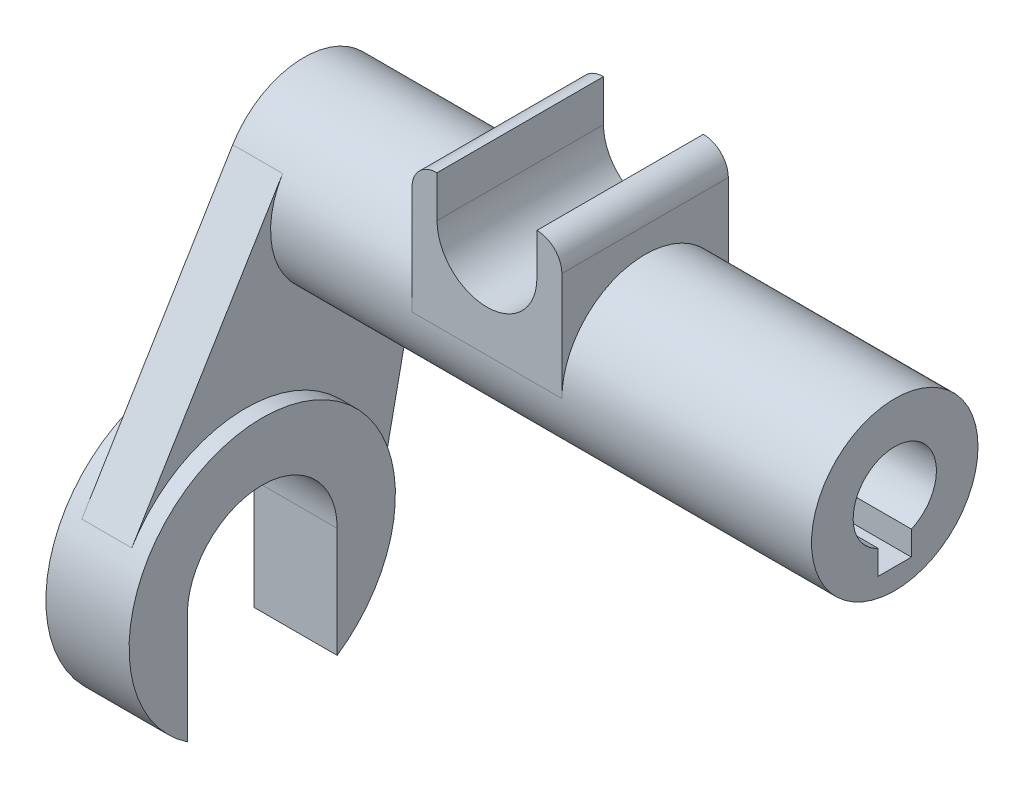
ISO-10303-21;
HEADER;
FILE_DESCRIPTION(('STEP AP214'),'2;1');
FILE_NAME('part.step','',(''),(''),'','','');
FILE_SCHEMA(('AUTOMOTIVE_DESIGN { 1 0 10303 214 1 1 1 1 }'));
ENDSEC;
DATA;
#1=APPLICATION_CONTEXT('core data for automotive mechanical design processes');
#2=APPLICATION_PROTOCOL_DEFINITION('international standard','automotive_design',2000,#1);
#3=PRODUCT_CONTEXT('',#1,'mechanical');
#4=PRODUCT('Part','Part','',(#3));
#5=PRODUCT_RELATED_PRODUCT_CATEGORY('part','',(#4));
#6=PRODUCT_DEFINITION_FORMATION('','',#4);
#7=PRODUCT_DEFINITION_CONTEXT('part definition',#1,'design');
#8=PRODUCT_DEFINITION('design','',#6,#7);
#9=PRODUCT_DEFINITION_SHAPE('','',#8);
#10=(LENGTH_UNIT() NAMED_UNIT(*) SI_UNIT(.MILLI.,.METRE.));
#11=(NAMED_UNIT(*) PLANE_ANGLE_UNIT() SI_UNIT($,.RADIAN.));
#12=(NAMED_UNIT(*) SI_UNIT($,.STERADIAN.) SOLID_ANGLE_UNIT());
#13=UNCERTAINTY_MEASURE_WITH_UNIT(LENGTH_MEASURE(1.E-05),#10,'distance_accuracy_value','');
#14=(GEOMETRIC_REPRESENTATION_CONTEXT(3) GLOBAL_UNCERTAINTY_ASSIGNED_CONTEXT((#13)) GLOBAL_UNIT_ASSIGNED_CONTEXT((#10,
#11,#12)) REPRESENTATION_CONTEXT('',''));
#15=CARTESIAN_POINT('',(0.,0.,0.));
#16=DIRECTION('',(0.,0.,1.));
#17=DIRECTION('',(1.,0.,0.));
#18=AXIS2_PLACEMENT_3D('',#15,#16,#17);
#19=CARTESIAN_POINT('',(71.,0.,0.));
#20=DIRECTION('',(-1.,0.,0.));
#21=DIRECTION('',(0.,0.,1.));
#22=AXIS2_PLACEMENT_3D('',#19,#20,#21);
#23=CYLINDRICAL_SURFACE('',#22,10.);
#24=CARTESIAN_POINT('',(6.,0.,0.));
#25=DIRECTION('',(-1.,0.,0.));
#26=DIRECTION('',(0.,0.,1.));
#27=AXIS2_PLACEMENT_3D('',#24,#25,#26);
#28=CIRCLE('',#27,10.);
#29=CARTESIAN_POINT('',(6.00000000000001,-2.03849376483833,-9.79002263382038));
#30=VERTEX_POINT('',#29);
#31=CARTESIAN_POINT('',(6.00000000000001,5.18634750092736,8.54995904081561));
#32=VERTEX_POINT('',#31);
#33=EDGE_CURVE('E58',#30,#32,#28,.T.);
#34=ORIENTED_EDGE('',*,*,#33,.F.);
#35=DIRECTION('',(-1.,0.,0.));
#36=VECTOR('',#35,1.);
#37=CARTESIAN_POINT('',(6.,-2.03849376483833,-9.79002263382038));
#38=LINE('',#37,#36);
#39=CARTESIAN_POINT('',(0.,-2.03849376483833,-9.79002263382038));
#40=VERTEX_POINT('',#39);
#41=EDGE_CURVE('E281',#30,#40,#38,.T.);
#42=ORIENTED_EDGE('',*,*,#41,.T.);
#43=CARTESIAN_POINT('',(0.,0.,0.));
#44=DIRECTION('',(1.,0.,0.));
#45=DIRECTION('',(0.,0.,-1.));
#46=AXIS2_PLACEMENT_3D('',#43,#44,#45);
#47=CIRCLE('',#46,10.);
#48=CARTESIAN_POINT('',(0.,5.18634750092736,8.54995904081561));
#49=VERTEX_POINT('',#48);
#50=EDGE_CURVE('E278',#40,#49,#47,.T.);
#51=ORIENTED_EDGE('',*,*,#50,.T.);
#52=DIRECTION('',(-1.,0.,0.));
#53=VECTOR('',#52,1.);
#54=CARTESIAN_POINT('',(6.,5.18634750092736,8.54995904081561));
#55=LINE('',#54,#53);
#56=EDGE_CURVE('E57',#32,#49,#55,.T.);
#57=ORIENTED_EDGE('',*,*,#56,.F.);
#58=EDGE_LOOP('',(#34,#42,#51,#57));
#59=FACE_BOUND('',#58,.T.);
#60=CARTESIAN_POINT('',(71.,0.,0.));
#61=DIRECTION('',(1.,0.,0.));
#62=DIRECTION('',(0.,0.,-1.));
#63=AXIS2_PLACEMENT_3D('',#60,#61,#62);
#64=CIRCLE('',#63,10.);
#65=CARTESIAN_POINT('',(71.,0.,-10.));
#66=VERTEX_POINT('',#65);
#67=EDGE_CURVE('E207',#66,#66,#64,.T.);
#68=ORIENTED_EDGE('',*,*,#67,.F.);
#69=EDGE_LOOP('',(#68));
#70=FACE_BOUND('',#69,.T.);
#71=CARTESIAN_POINT('',(23.,0.,0.));
#72=DIRECTION('',(-1.,0.,0.));
#73=DIRECTION('',(0.,0.,-1.));
#74=AXIS2_PLACEMENT_3D('',#71,#72,#73);
#75=CIRCLE('',#74,10.);
#76=CARTESIAN_POINT('',(23.,0.,10.));
#77=VERTEX_POINT('',#76);
#78=CARTESIAN_POINT('',(23.,0.,-10.));
#79=VERTEX_POINT('',#78);
#80=EDGE_CURVE('E238',#77,#79,#75,.T.);
#81=ORIENTED_EDGE('',*,*,#80,.T.);
#82=DIRECTION('',(1.,0.,0.));
#83=VECTOR('',#82,1.);
#84=CARTESIAN_POINT('',(23.,0.,-10.));
#85=LINE('',#84,#83);
#86=CARTESIAN_POINT('',(41.,0.,-10.));
#87=VERTEX_POINT('',#86);
#88=EDGE_CURVE('E246',#79,#87,#85,.T.);
#89=ORIENTED_EDGE('',*,*,#88,.T.);
#90=CARTESIAN_POINT('',(41.,0.,0.));
#91=DIRECTION('',(-1.,0.,0.));
#92=DIRECTION('',(0.,0.,-1.));
#93=AXIS2_PLACEMENT_3D('',#90,#91,#92);
#94=CIRCLE('',#93,10.);
#95=CARTESIAN_POINT('',(41.,0.,10.));
#96=VERTEX_POINT('',#95);
#97=EDGE_CURVE('E228',#96,#87,#94,.T.);
#98=ORIENTED_EDGE('',*,*,#97,.F.);
#99=DIRECTION('',(1.,0.,0.));
#100=VECTOR('',#99,1.);
#101=CARTESIAN_POINT('',(23.,0.,10.));
#102=LINE('',#101,#100);
#103=EDGE_CURVE('E240',#77,#96,#102,.T.);
#104=ORIENTED_EDGE('',*,*,#103,.F.);
#105=EDGE_LOOP('',(#81,#89,#98,#104));
#106=FACE_BOUND('',#105,.T.);
#107=ADVANCED_FACE('F41',(#59,#70,#106),#23,.T.);
#108=CARTESIAN_POINT('',(71.,0.,0.));
#109=DIRECTION('',(1.,0.,0.));
#110=DIRECTION('',(0.,0.,-1.));
#111=AXIS2_PLACEMENT_3D('',#108,#109,#110);
#112=PLANE('',#111);
#113=CARTESIAN_POINT('',(71.,0.,0.));
#114=DIRECTION('',(1.,0.,0.));
#115=DIRECTION('',(0.,0.,-1.));
#116=AXIS2_PLACEMENT_3D('',#113,#114,#115);
#117=CIRCLE('',#116,5.);
#118=CARTESIAN_POINT('',(71.,-4.58257569495584,-2.));
#119=VERTEX_POINT('',#118);
#120=CARTESIAN_POINT('',(71.,-4.58257569495584,2.));
#121=VERTEX_POINT('',#120);
#122=EDGE_CURVE('E256',#119,#121,#117,.T.);
#123=ORIENTED_EDGE('',*,*,#122,.F.);
#124=DIRECTION('',(0.,1.,0.));
#125=VECTOR('',#124,1.);
#126=CARTESIAN_POINT('',(71.,-7.5,-2.));
#127=LINE('',#126,#125);
#128=CARTESIAN_POINT('',(71.,-7.5,-2.));
#129=VERTEX_POINT('',#128);
#130=EDGE_CURVE('E262',#129,#119,#127,.T.);
#131=ORIENTED_EDGE('',*,*,#130,.F.);
#132=DIRECTION('',(0.,0.,-1.));
#133=VECTOR('',#132,1.);
#134=CARTESIAN_POINT('',(71.,-7.5,2.));
#135=LINE('',#134,#133);
#136=CARTESIAN_POINT('',(71.,-7.5,2.));
#137=VERTEX_POINT('',#136);
#138=EDGE_CURVE('E263',#137,#129,#135,.T.);
#139=ORIENTED_EDGE('',*,*,#138,.F.);
#140=DIRECTION('',(0.,-1.,0.));
#141=VECTOR('',#140,1.);
#142=CARTESIAN_POINT('',(71.,-4.58257569495584,2.));
#143=LINE('',#142,#141);
#144=EDGE_CURVE('E257',#121,#137,#143,.T.);
#145=ORIENTED_EDGE('',*,*,#144,.F.);
#146=EDGE_LOOP('',(#123,#131,#139,#145));
#147=FACE_BOUND('',#146,.T.);
#148=ORIENTED_EDGE('',*,*,#67,.T.);
#149=EDGE_LOOP('',(#148));
#150=FACE_BOUND('',#149,.T.);
#151=ADVANCED_FACE('F325',(#147,#150),#112,.T.);
#152=CARTESIAN_POINT('',(0.,0.,0.));
#153=DIRECTION('',(1.,0.,0.));
#154=DIRECTION('',(0.,0.,-1.));
#155=AXIS2_PLACEMENT_3D('',#152,#153,#154);
#156=PLANE('',#155);
#157=DIRECTION('',(0.,-1.,0.));
#158=VECTOR('',#157,1.);
#159=CARTESIAN_POINT('',(0.,-7.5,-2.));
#160=LINE('',#159,#158);
#161=CARTESIAN_POINT('',(0.,-4.58257569495584,-2.));
#162=VERTEX_POINT('',#161);
#163=CARTESIAN_POINT('',(0.,-7.5,-2.));
#164=VERTEX_POINT('',#163);
#165=EDGE_CURVE('E249',#162,#164,#160,.T.);
#166=ORIENTED_EDGE('',*,*,#165,.F.);
#167=CARTESIAN_POINT('',(0.,0.,0.));
#168=DIRECTION('',(1.,0.,0.));
#169=DIRECTION('',(0.,0.,-1.));
#170=AXIS2_PLACEMENT_3D('',#167,#168,#169);
#171=CIRCLE('',#170,5.);
#172=CARTESIAN_POINT('',(0.,-4.58257569495584,2.));
#173=VERTEX_POINT('',#172);
#174=EDGE_CURVE('E254',#173,#162,#171,.F.);
#175=ORIENTED_EDGE('',*,*,#174,.F.);
#176=DIRECTION('',(0.,1.,0.));
#177=VECTOR('',#176,1.);
#178=CARTESIAN_POINT('',(0.,-4.58257569495584,2.));
#179=LINE('',#178,#177);
#180=CARTESIAN_POINT('',(0.,-7.5,2.));
#181=VERTEX_POINT('',#180);
#182=EDGE_CURVE('E267',#181,#173,#179,.T.);
#183=ORIENTED_EDGE('',*,*,#182,.F.);
#184=DIRECTION('',(0.,0.,1.));
#185=VECTOR('',#184,1.);
#186=CARTESIAN_POINT('',(0.,-7.5,2.));
#187=LINE('',#186,#185);
#188=EDGE_CURVE('E244',#164,#181,#187,.T.);
#189=ORIENTED_EDGE('',*,*,#188,.F.);
#190=EDGE_LOOP('',(#166,#175,#183,#189));
#191=FACE_BOUND('',#190,.T.);
#192=ORIENTED_EDGE('',*,*,#50,.F.);
#193=DIRECTION('',(0.,0.979002263382038,-0.203849376483833));
#194=VECTOR('',#193,1.);
#195=CARTESIAN_POINT('',(0.,-2.03849376483833,-9.79002263382038));
#196=LINE('',#195,#194);
#197=CARTESIAN_POINT('',(0.,-36.2615900237413,-2.6640362141126));
#198=VERTEX_POINT('',#197);
#199=EDGE_CURVE('E301',#198,#40,#196,.T.);
#200=ORIENTED_EDGE('',*,*,#199,.F.);
#201=CARTESIAN_POINT('',(0.,-33.,13.));
#202=DIRECTION('',(-1.,0.,0.));
#203=DIRECTION('',(0.,0.,1.));
#204=AXIS2_PLACEMENT_3D('',#201,#202,#203);
#205=CIRCLE('',#204,16.);
#206=CARTESIAN_POINT('',(0.,-24.7018439985162,26.679934465305));
#207=VERTEX_POINT('',#206);
#208=EDGE_CURVE('E297',#207,#198,#205,.T.);
#209=ORIENTED_EDGE('',*,*,#208,.F.);
#210=DIRECTION('',(0.,0.854995904081561,-0.518634750092736));
#211=VECTOR('',#210,1.);
#212=CARTESIAN_POINT('',(0.,5.18634750092736,8.5499590408156));
#213=LINE('',#212,#211);
#214=EDGE_CURVE('E291',#207,#49,#213,.T.);
#215=ORIENTED_EDGE('',*,*,#214,.T.);
#216=EDGE_LOOP('',(#192,#200,#209,#215));
#217=FACE_BOUND('',#216,.T.);
#218=ADVANCED_FACE('F299',(#191,#217),#156,.F.);
#219=CARTESIAN_POINT('',(-0.001000000000001,0.,0.));
#220=DIRECTION('',(1.,0.,0.));
#221=DIRECTION('',(0.,0.,-1.));
#222=AXIS2_PLACEMENT_3D('',#219,#220,#221);
#223=CYLINDRICAL_SURFACE('',#222,5.);
#224=ORIENTED_EDGE('',*,*,#174,.T.);
#225=DIRECTION('',(1.,0.,0.));
#226=VECTOR('',#225,1.);
#227=CARTESIAN_POINT('',(-0.001000000000001,-4.58257569495584,-2.));
#228=LINE('',#227,#226);
#229=EDGE_CURVE('E266',#162,#119,#228,.T.);
#230=ORIENTED_EDGE('',*,*,#229,.T.);
#231=ORIENTED_EDGE('',*,*,#122,.T.);
#232=DIRECTION('',(1.,0.,0.));
#233=VECTOR('',#232,1.);
#234=CARTESIAN_POINT('',(-0.001000000000001,-4.58257569495584,2.));
#235=LINE('',#234,#233);
#236=EDGE_CURVE('E270',#173,#121,#235,.T.);
#237=ORIENTED_EDGE('',*,*,#236,.F.);
#238=EDGE_LOOP('',(#224,#230,#231,#237));
#239=FACE_BOUND('',#238,.T.);
#240=ADVANCED_FACE('F351',(#239),#223,.F.);
#241=CARTESIAN_POINT('',(-0.001000000000001,-7.5,-2.));
#242=DIRECTION('',(0.,0.,-1.));
#243=DIRECTION('',(0.,1.,0.));
#244=AXIS2_PLACEMENT_3D('',#241,#242,#243);
#245=PLANE('',#244);
#246=ORIENTED_EDGE('',*,*,#165,.T.);
#247=DIRECTION('',(1.,0.,0.));
#248=VECTOR('',#247,1.);
#249=CARTESIAN_POINT('',(-0.001000000000001,-7.5,-2.));
#250=LINE('',#249,#248);
#251=EDGE_CURVE('E272',#164,#129,#250,.T.);
#252=ORIENTED_EDGE('',*,*,#251,.T.);
#253=ORIENTED_EDGE('',*,*,#130,.T.);
#254=ORIENTED_EDGE('',*,*,#229,.F.);
#255=EDGE_LOOP('',(#246,#252,#253,#254));
#256=FACE_BOUND('',#255,.T.);
#257=ADVANCED_FACE('F347',(#256),#245,.F.);
#258=CARTESIAN_POINT('',(-0.001000000000001,-7.5,2.));
#259=DIRECTION('',(0.,-1.,0.));
#260=DIRECTION('',(0.,0.,-1.));
#261=AXIS2_PLACEMENT_3D('',#258,#259,#260);
#262=PLANE('',#261);
#263=ORIENTED_EDGE('',*,*,#188,.T.);
#264=DIRECTION('',(1.,0.,0.));
#265=VECTOR('',#264,1.);
#266=CARTESIAN_POINT('',(-0.001000000000001,-7.5,2.));
#267=LINE('',#266,#265);
#268=EDGE_CURVE('E271',#181,#137,#267,.T.);
#269=ORIENTED_EDGE('',*,*,#268,.T.);
#270=ORIENTED_EDGE('',*,*,#138,.T.);
#271=ORIENTED_EDGE('',*,*,#251,.F.);
#272=EDGE_LOOP('',(#263,#269,#270,#271));
#273=FACE_BOUND('',#272,.T.);
#274=ADVANCED_FACE('F355',(#273),#262,.F.);
#275=CARTESIAN_POINT('',(-0.001000000000001,-4.58257569495584,2.));
#276=DIRECTION('',(0.,0.,1.));
#277=DIRECTION('',(0.,-1.,0.));
#278=AXIS2_PLACEMENT_3D('',#275,#276,#277);
#279=PLANE('',#278);
#280=ORIENTED_EDGE('',*,*,#182,.T.);
#281=ORIENTED_EDGE('',*,*,#236,.T.);
#282=ORIENTED_EDGE('',*,*,#144,.T.);
#283=ORIENTED_EDGE('',*,*,#268,.F.);
#284=EDGE_LOOP('',(#280,#281,#282,#283));
#285=FACE_BOUND('',#284,.T.);
#286=ADVANCED_FACE('F350',(#285),#279,.F.);
#287=CARTESIAN_POINT('',(23.,0.,10.));
#288=DIRECTION('',(0.,0.,1.));
#289=DIRECTION('',(1.,0.,0.));
#290=AXIS2_PLACEMENT_3D('',#287,#288,#289);
#291=PLANE('',#290);
#292=DIRECTION('',(0.,1.,0.));
#293=VECTOR('',#292,1.);
#294=CARTESIAN_POINT('',(38.,0.,10.));
#295=LINE('',#294,#293);
#296=CARTESIAN_POINT('',(38.,11.01,10.));
#297=VERTEX_POINT('',#296);
#298=CARTESIAN_POINT('',(38.,16.,10.));
#299=VERTEX_POINT('',#298);
#300=EDGE_CURVE('E234',#297,#299,#295,.T.);
#301=ORIENTED_EDGE('',*,*,#300,.F.);
#302=CARTESIAN_POINT('',(32.,11.01,10.));
#303=DIRECTION('',(0.,0.,1.));
#304=DIRECTION('',(1.,0.,0.));
#305=AXIS2_PLACEMENT_3D('',#302,#303,#304);
#306=CIRCLE('',#305,6.);
#307=CARTESIAN_POINT('',(26.,11.01,10.));
#308=VERTEX_POINT('',#307);
#309=EDGE_CURVE('E520',#308,#297,#306,.T.);
#310=ORIENTED_EDGE('',*,*,#309,.F.);
#311=DIRECTION('',(0.,-1.,0.));
#312=VECTOR('',#311,1.);
#313=CARTESIAN_POINT('',(26.,0.,10.));
#314=LINE('',#313,#312);
#315=CARTESIAN_POINT('',(26.,16.,10.));
#316=VERTEX_POINT('',#315);
#317=EDGE_CURVE('E523',#316,#308,#314,.T.);
#318=ORIENTED_EDGE('',*,*,#317,.F.);
#319=CARTESIAN_POINT('',(26.,13.,10.));
#320=DIRECTION('',(0.,0.,1.));
#321=DIRECTION('',(1.,0.,0.));
#322=AXIS2_PLACEMENT_3D('',#319,#320,#321);
#323=CIRCLE('',#322,3.);
#324=CARTESIAN_POINT('',(23.,13.,10.));
#325=VERTEX_POINT('',#324);
#326=EDGE_CURVE('E199',#316,#325,#323,.T.);
#327=ORIENTED_EDGE('',*,*,#326,.T.);
#328=DIRECTION('',(0.,-1.,0.));
#329=VECTOR('',#328,1.);
#330=CARTESIAN_POINT('',(23.,0.,10.));
#331=LINE('',#330,#329);
#332=EDGE_CURVE('E247',#325,#77,#331,.T.);
#333=ORIENTED_EDGE('',*,*,#332,.T.);
#334=ORIENTED_EDGE('',*,*,#103,.T.);
#335=DIRECTION('',(0.,-1.,0.));
#336=VECTOR('',#335,1.);
#337=CARTESIAN_POINT('',(41.,0.,10.));
#338=LINE('',#337,#336);
#339=CARTESIAN_POINT('',(41.,13.,10.));
#340=VERTEX_POINT('',#339);
#341=EDGE_CURVE('E226',#340,#96,#338,.T.);
#342=ORIENTED_EDGE('',*,*,#341,.F.);
#343=CARTESIAN_POINT('',(38.,13.,10.));
#344=DIRECTION('',(0.,0.,1.));
#345=DIRECTION('',(1.,0.,0.));
#346=AXIS2_PLACEMENT_3D('',#343,#344,#345);
#347=CIRCLE('',#346,3.);
#348=EDGE_CURVE('E203',#340,#299,#347,.T.);
#349=ORIENTED_EDGE('',*,*,#348,.T.);
#350=EDGE_LOOP('',(#301,#310,#318,#327,#333,#334,#342,#349));
#351=FACE_BOUND('',#350,.T.);
#352=ADVANCED_FACE('F235',(#351),#291,.T.);
#353=CARTESIAN_POINT('',(23.,16.,-10.));
#354=DIRECTION('',(0.,0.,-1.));
#355=DIRECTION('',(-1.,0.,0.));
#356=AXIS2_PLACEMENT_3D('',#353,#354,#355);
#357=PLANE('',#356);
#358=DIRECTION('',(0.,1.,0.));
#359=VECTOR('',#358,1.);
#360=CARTESIAN_POINT('',(38.,11.01,-10.));
#361=LINE('',#360,#359);
#362=CARTESIAN_POINT('',(38.,11.01,-10.));
#363=VERTEX_POINT('',#362);
#364=CARTESIAN_POINT('',(38.,16.,-10.));
#365=VERTEX_POINT('',#364);
#366=EDGE_CURVE('E216',#363,#365,#361,.T.);
#367=ORIENTED_EDGE('',*,*,#366,.T.);
#368=CARTESIAN_POINT('',(38.,13.,-10.));
#369=DIRECTION('',(0.,0.,-1.));
#370=DIRECTION('',(-1.,0.,0.));
#371=AXIS2_PLACEMENT_3D('',#368,#369,#370);
#372=CIRCLE('',#371,3.);
#373=CARTESIAN_POINT('',(41.,13.,-10.));
#374=VERTEX_POINT('',#373);
#375=EDGE_CURVE('E200',#365,#374,#372,.T.);
#376=ORIENTED_EDGE('',*,*,#375,.T.);
#377=DIRECTION('',(0.,1.,0.));
#378=VECTOR('',#377,1.);
#379=CARTESIAN_POINT('',(41.,16.,-10.));
#380=LINE('',#379,#378);
#381=EDGE_CURVE('E214',#87,#374,#380,.T.);
#382=ORIENTED_EDGE('',*,*,#381,.F.);
#383=ORIENTED_EDGE('',*,*,#88,.F.);
#384=DIRECTION('',(0.,1.,0.));
#385=VECTOR('',#384,1.);
#386=CARTESIAN_POINT('',(23.,16.,-10.));
#387=LINE('',#386,#385);
#388=CARTESIAN_POINT('',(23.,13.,-10.));
#389=VERTEX_POINT('',#388);
#390=EDGE_CURVE('E193',#79,#389,#387,.T.);
#391=ORIENTED_EDGE('',*,*,#390,.T.);
#392=CARTESIAN_POINT('',(26.,13.,-10.));
#393=DIRECTION('',(0.,0.,-1.));
#394=DIRECTION('',(-1.,0.,0.));
#395=AXIS2_PLACEMENT_3D('',#392,#393,#394);
#396=CIRCLE('',#395,3.);
#397=CARTESIAN_POINT('',(26.,16.,-10.));
#398=VERTEX_POINT('',#397);
#399=EDGE_CURVE('E47',#389,#398,#396,.T.);
#400=ORIENTED_EDGE('',*,*,#399,.T.);
#401=DIRECTION('',(0.,-1.,0.));
#402=VECTOR('',#401,1.);
#403=CARTESIAN_POINT('',(26.,16.,-10.));
#404=LINE('',#403,#402);
#405=CARTESIAN_POINT('',(26.,11.01,-10.));
#406=VERTEX_POINT('',#405);
#407=EDGE_CURVE('E176',#398,#406,#404,.T.);
#408=ORIENTED_EDGE('',*,*,#407,.T.);
#409=CARTESIAN_POINT('',(32.,11.01,-10.));
#410=DIRECTION('',(0.,0.,1.));
#411=DIRECTION('',(1.,0.,0.));
#412=AXIS2_PLACEMENT_3D('',#409,#410,#411);
#413=CIRCLE('',#412,6.);
#414=EDGE_CURVE('E190',#406,#363,#413,.T.);
#415=ORIENTED_EDGE('',*,*,#414,.T.);
#416=EDGE_LOOP('',(#367,#376,#382,#383,#391,#400,#408,#415));
#417=FACE_BOUND('',#416,.T.);
#418=ADVANCED_FACE('F195',(#417),#357,.T.);
#419=CARTESIAN_POINT('',(23.,0.,0.));
#420=DIRECTION('',(1.,0.,0.));
#421=DIRECTION('',(0.,0.,-1.));
#422=AXIS2_PLACEMENT_3D('',#419,#420,#421);
#423=PLANE('',#422);
#424=ORIENTED_EDGE('',*,*,#332,.F.);
#425=DIRECTION('',(0.,0.,1.));
#426=VECTOR('',#425,1.);
#427=CARTESIAN_POINT('',(23.,13.,-10.));
#428=LINE('',#427,#426);
#429=EDGE_CURVE('E211',#325,#389,#428,.F.);
#430=ORIENTED_EDGE('',*,*,#429,.T.);
#431=ORIENTED_EDGE('',*,*,#390,.F.);
#432=ORIENTED_EDGE('',*,*,#80,.F.);
#433=EDGE_LOOP('',(#424,#430,#431,#432));
#434=FACE_BOUND('',#433,.T.);
#435=ADVANCED_FACE('F316',(#434),#423,.F.);
#436=CARTESIAN_POINT('',(41.,0.,0.));
#437=DIRECTION('',(1.,0.,0.));
#438=DIRECTION('',(0.,0.,-1.));
#439=AXIS2_PLACEMENT_3D('',#436,#437,#438);
#440=PLANE('',#439);
#441=ORIENTED_EDGE('',*,*,#381,.T.);
#442=DIRECTION('',(0.,0.,1.));
#443=VECTOR('',#442,1.);
#444=CARTESIAN_POINT('',(41.,13.,0.));
#445=LINE('',#444,#443);
#446=EDGE_CURVE('E11',#374,#340,#445,.T.);
#447=ORIENTED_EDGE('',*,*,#446,.T.);
#448=ORIENTED_EDGE('',*,*,#341,.T.);
#449=ORIENTED_EDGE('',*,*,#97,.T.);
#450=EDGE_LOOP('',(#441,#447,#448,#449));
#451=FACE_BOUND('',#450,.T.);
#452=ADVANCED_FACE('F221',(#451),#440,.T.);
#453=CARTESIAN_POINT('',(26.,13.,10.));
#454=DIRECTION('',(0.,0.,-1.));
#455=DIRECTION('',(-1.,0.,0.));
#456=AXIS2_PLACEMENT_3D('',#453,#454,#455);
#457=CYLINDRICAL_SURFACE('',#456,3.);
#458=ORIENTED_EDGE('',*,*,#399,.F.);
#459=ORIENTED_EDGE('',*,*,#429,.F.);
#460=ORIENTED_EDGE('',*,*,#326,.F.);
#461=DIRECTION('',(0.,0.,1.));
#462=VECTOR('',#461,1.);
#463=CARTESIAN_POINT('',(26.,16.,10.));
#464=LINE('',#463,#462);
#465=EDGE_CURVE('E179',#398,#316,#464,.T.);
#466=ORIENTED_EDGE('',*,*,#465,.F.);
#467=EDGE_LOOP('',(#458,#459,#460,#466));
#468=FACE_BOUND('',#467,.T.);
#469=ADVANCED_FACE('F197',(#468),#457,.T.);
#470=CARTESIAN_POINT('',(38.,13.,0.));
#471=DIRECTION('',(0.,0.,1.));
#472=DIRECTION('',(1.,0.,0.));
#473=AXIS2_PLACEMENT_3D('',#470,#471,#472);
#474=CYLINDRICAL_SURFACE('',#473,3.);
#475=ORIENTED_EDGE('',*,*,#375,.F.);
#476=DIRECTION('',(0.,0.,1.));
#477=VECTOR('',#476,1.);
#478=CARTESIAN_POINT('',(38.,16.,10.));
#479=LINE('',#478,#477);
#480=EDGE_CURVE('E205',#299,#365,#479,.F.);
#481=ORIENTED_EDGE('',*,*,#480,.F.);
#482=ORIENTED_EDGE('',*,*,#348,.F.);
#483=ORIENTED_EDGE('',*,*,#446,.F.);
#484=EDGE_LOOP('',(#475,#481,#482,#483));
#485=FACE_BOUND('',#484,.T.);
#486=ADVANCED_FACE('F43',(#485),#474,.T.);
#487=CARTESIAN_POINT('',(6.,-2.03849376483833,-9.79002263382038));
#488=DIRECTION('',(0.,0.203849376483833,0.979002263382038));
#489=DIRECTION('',(0.,-0.979002263382038,0.203849376483833));
#490=AXIS2_PLACEMENT_3D('',#487,#488,#489);
#491=PLANE('',#490);
#492=ORIENTED_EDGE('',*,*,#199,.T.);
#493=ORIENTED_EDGE('',*,*,#41,.F.);
#494=DIRECTION('',(0.,0.979002263382038,-0.203849376483833));
#495=VECTOR('',#494,1.);
#496=CARTESIAN_POINT('',(6.,-2.03849376483833,-9.79002263382038));
#497=LINE('',#496,#495);
#498=CARTESIAN_POINT('',(6.,-36.2615900237413,-2.6640362141126));
#499=VERTEX_POINT('',#498);
#500=EDGE_CURVE('E312',#499,#30,#497,.T.);
#501=ORIENTED_EDGE('',*,*,#500,.F.);
#502=DIRECTION('',(-1.,0.,0.));
#503=VECTOR('',#502,1.);
#504=CARTESIAN_POINT('',(6.,-36.2615900237413,-2.6640362141126));
#505=LINE('',#504,#503);
#506=EDGE_CURVE('E307',#499,#198,#505,.T.);
#507=ORIENTED_EDGE('',*,*,#506,.T.);
#508=EDGE_LOOP('',(#492,#493,#501,#507));
#509=FACE_BOUND('',#508,.T.);
#510=ADVANCED_FACE('F340',(#509),#491,.F.);
#511=CARTESIAN_POINT('',(6.,5.18634750092736,8.5499590408156));
#512=DIRECTION('',(0.,0.518634750092736,0.85499590408156));
#513=DIRECTION('',(0.,-0.854995904081561,0.518634750092736));
#514=AXIS2_PLACEMENT_3D('',#511,#512,#513);
#515=PLANE('',#514);
#516=ORIENTED_EDGE('',*,*,#214,.F.);
#517=DIRECTION('',(-1.,0.,0.));
#518=VECTOR('',#517,1.);
#519=CARTESIAN_POINT('',(6.,-24.7018439985162,26.679934465305));
#520=LINE('',#519,#518);
#521=CARTESIAN_POINT('',(6.,-24.7018439985162,26.679934465305));
#522=VERTEX_POINT('',#521);
#523=EDGE_CURVE('E298',#522,#207,#520,.T.);
#524=ORIENTED_EDGE('',*,*,#523,.F.);
#525=DIRECTION('',(0.,0.854995904081561,-0.518634750092736));
#526=VECTOR('',#525,1.);
#527=CARTESIAN_POINT('',(6.,5.18634750092736,8.5499590408156));
#528=LINE('',#527,#526);
#529=EDGE_CURVE('E294',#522,#32,#528,.T.);
#530=ORIENTED_EDGE('',*,*,#529,.T.);
#531=ORIENTED_EDGE('',*,*,#56,.T.);
#532=EDGE_LOOP('',(#516,#524,#530,#531));
#533=FACE_BOUND('',#532,.T.);
#534=ADVANCED_FACE('F293',(#533),#515,.T.);
#535=CARTESIAN_POINT('',(6.,0.,0.));
#536=DIRECTION('',(-1.,0.,0.));
#537=DIRECTION('',(0.,0.,1.));
#538=AXIS2_PLACEMENT_3D('',#535,#536,#537);
#539=PLANE('',#538);
#540=CARTESIAN_POINT('',(6.,-33.,13.));
#541=DIRECTION('',(-1.,0.,0.));
#542=DIRECTION('',(0.,0.,1.));
#543=AXIS2_PLACEMENT_3D('',#540,#541,#542);
#544=CIRCLE('',#543,16.);
#545=EDGE_CURVE('E303',#522,#499,#544,.T.);
#546=ORIENTED_EDGE('',*,*,#545,.T.);
#547=ORIENTED_EDGE('',*,*,#500,.T.);
#548=ORIENTED_EDGE('',*,*,#33,.T.);
#549=ORIENTED_EDGE('',*,*,#529,.F.);
#550=EDGE_LOOP('',(#546,#547,#548,#549));
#551=FACE_BOUND('',#550,.T.);
#552=ADVANCED_FACE('F394',(#551),#539,.F.);
#553=CARTESIAN_POINT('',(-2.,-33.,13.));
#554=DIRECTION('',(1.,0.,0.));
#555=DIRECTION('',(0.,0.,-1.));
#556=AXIS2_PLACEMENT_3D('',#553,#554,#555);
#557=CYLINDRICAL_SURFACE('',#556,16.);
#558=DIRECTION('',(1.,0.,0.));
#559=VECTOR('',#558,1.);
#560=CARTESIAN_POINT('',(-2.,-46.228756555323,22.));
#561=LINE('',#560,#559);
#562=CARTESIAN_POINT('',(-2.,-46.228756555323,22.));
#563=VERTEX_POINT('',#562);
#564=CARTESIAN_POINT('',(8.,-46.228756555323,22.));
#565=VERTEX_POINT('',#564);
#566=EDGE_CURVE('E547',#563,#565,#561,.T.);
#567=ORIENTED_EDGE('',*,*,#566,.T.);
#568=CARTESIAN_POINT('',(8.,-33.,13.));
#569=DIRECTION('',(-1.,0.,0.));
#570=DIRECTION('',(0.,0.,1.));
#571=AXIS2_PLACEMENT_3D('',#568,#569,#570);
#572=CIRCLE('',#571,16.);
#573=CARTESIAN_POINT('',(8.,-46.228756555323,4.00000000000001));
#574=VERTEX_POINT('',#573);
#575=EDGE_CURVE('E519',#565,#574,#572,.T.);
#576=ORIENTED_EDGE('',*,*,#575,.T.);
#577=DIRECTION('',(1.,0.,0.));
#578=VECTOR('',#577,1.);
#579=CARTESIAN_POINT('',(-2.,-46.228756555323,4.00000000000001));
#580=LINE('',#579,#578);
#581=CARTESIAN_POINT('',(-2.,-46.228756555323,4.00000000000001));
#582=VERTEX_POINT('',#581);
#583=EDGE_CURVE('E304',#582,#574,#580,.T.);
#584=ORIENTED_EDGE('',*,*,#583,.F.);
#585=CARTESIAN_POINT('',(-2.,-33.,13.));
#586=DIRECTION('',(-1.,0.,0.));
#587=DIRECTION('',(0.,0.,1.));
#588=AXIS2_PLACEMENT_3D('',#585,#586,#587);
#589=CIRCLE('',#588,16.);
#590=EDGE_CURVE('E543',#563,#582,#589,.T.);
#591=ORIENTED_EDGE('',*,*,#590,.F.);
#592=EDGE_LOOP('',(#567,#576,#584,#591));
#593=FACE_BOUND('',#592,.T.);
#594=ORIENTED_EDGE('',*,*,#523,.T.);
#595=ORIENTED_EDGE('',*,*,#208,.T.);
#596=ORIENTED_EDGE('',*,*,#506,.F.);
#597=ORIENTED_EDGE('',*,*,#545,.F.);
#598=EDGE_LOOP('',(#594,#595,#596,#597));
#599=FACE_BOUND('',#598,.T.);
#600=ADVANCED_FACE('F405',(#593,#599),#557,.T.);
#601=CARTESIAN_POINT('',(-2.,-33.,4.));
#602=DIRECTION('',(0.,0.,-1.));
#603=DIRECTION('',(0.,1.,0.));
#604=AXIS2_PLACEMENT_3D('',#601,#602,#603);
#605=PLANE('',#604);
#606=ORIENTED_EDGE('',*,*,#583,.T.);
#607=DIRECTION('',(0.,1.,0.));
#608=VECTOR('',#607,1.);
#609=CARTESIAN_POINT('',(8.,-33.,4.));
#610=LINE('',#609,#608);
#611=CARTESIAN_POINT('',(8.,-33.,4.));
#612=VERTEX_POINT('',#611);
#613=EDGE_CURVE('E535',#574,#612,#610,.T.);
#614=ORIENTED_EDGE('',*,*,#613,.T.);
#615=DIRECTION('',(1.,0.,0.));
#616=VECTOR('',#615,1.);
#617=CARTESIAN_POINT('',(-2.,-33.,4.));
#618=LINE('',#617,#616);
#619=CARTESIAN_POINT('',(-2.,-33.,4.));
#620=VERTEX_POINT('',#619);
#621=EDGE_CURVE('E555',#620,#612,#618,.T.);
#622=ORIENTED_EDGE('',*,*,#621,.F.);
#623=DIRECTION('',(0.,1.,0.));
#624=VECTOR('',#623,1.);
#625=CARTESIAN_POINT('',(-2.,-33.,4.));
#626=LINE('',#625,#624);
#627=EDGE_CURVE('E542',#582,#620,#626,.T.);
#628=ORIENTED_EDGE('',*,*,#627,.F.);
#629=EDGE_LOOP('',(#606,#614,#622,#628));
#630=FACE_BOUND('',#629,.T.);
#631=ADVANCED_FACE('F415',(#630),#605,.F.);
#632=CARTESIAN_POINT('',(-2.,-33.,13.));
#633=DIRECTION('',(1.,0.,0.));
#634=DIRECTION('',(0.,0.,-1.));
#635=AXIS2_PLACEMENT_3D('',#632,#633,#634);
#636=CYLINDRICAL_SURFACE('',#635,9.);
#637=ORIENTED_EDGE('',*,*,#621,.T.);
#638=CARTESIAN_POINT('',(8.,-33.,13.));
#639=DIRECTION('',(1.,0.,0.));
#640=DIRECTION('',(0.,0.,1.));
#641=AXIS2_PLACEMENT_3D('',#638,#639,#640);
#642=CIRCLE('',#641,9.);
#643=CARTESIAN_POINT('',(8.,-33.,22.));
#644=VERTEX_POINT('',#643);
#645=EDGE_CURVE('E533',#612,#644,#642,.T.);
#646=ORIENTED_EDGE('',*,*,#645,.T.);
#647=DIRECTION('',(1.,0.,0.));
#648=VECTOR('',#647,1.);
#649=CARTESIAN_POINT('',(-2.,-33.,22.));
#650=LINE('',#649,#648);
#651=CARTESIAN_POINT('',(-2.,-33.,22.));
#652=VERTEX_POINT('',#651);
#653=EDGE_CURVE('E552',#652,#644,#650,.T.);
#654=ORIENTED_EDGE('',*,*,#653,.F.);
#655=CARTESIAN_POINT('',(-2.,-33.,13.));
#656=DIRECTION('',(1.,0.,0.));
#657=DIRECTION('',(0.,0.,1.));
#658=AXIS2_PLACEMENT_3D('',#655,#656,#657);
#659=CIRCLE('',#658,9.);
#660=EDGE_CURVE('E548',#620,#652,#659,.T.);
#661=ORIENTED_EDGE('',*,*,#660,.F.);
#662=EDGE_LOOP('',(#637,#646,#654,#661));
#663=FACE_BOUND('',#662,.T.);
#664=ADVANCED_FACE('F421',(#663),#636,.F.);
#665=CARTESIAN_POINT('',(-2.,-33.,22.));
#666=DIRECTION('',(0.,0.,1.));
#667=DIRECTION('',(1.,0.,0.));
#668=AXIS2_PLACEMENT_3D('',#665,#666,#667);
#669=PLANE('',#668);
#670=ORIENTED_EDGE('',*,*,#653,.T.);
#671=DIRECTION('',(0.,-1.,0.));
#672=VECTOR('',#671,1.);
#673=CARTESIAN_POINT('',(8.,-33.,22.));
#674=LINE('',#673,#672);
#675=EDGE_CURVE('E537',#644,#565,#674,.T.);
#676=ORIENTED_EDGE('',*,*,#675,.T.);
#677=ORIENTED_EDGE('',*,*,#566,.F.);
#678=DIRECTION('',(0.,-1.,0.));
#679=VECTOR('',#678,1.);
#680=CARTESIAN_POINT('',(-2.,-33.,22.));
#681=LINE('',#680,#679);
#682=EDGE_CURVE('E546',#652,#563,#681,.T.);
#683=ORIENTED_EDGE('',*,*,#682,.F.);
#684=EDGE_LOOP('',(#670,#676,#677,#683));
#685=FACE_BOUND('',#684,.T.);
#686=ADVANCED_FACE('F427',(#685),#669,.F.);
#687=CARTESIAN_POINT('',(-2.,-33.,13.));
#688=DIRECTION('',(-1.,0.,0.));
#689=DIRECTION('',(0.,0.,1.));
#690=AXIS2_PLACEMENT_3D('',#687,#688,#689);
#691=PLANE('',#690);
#692=ORIENTED_EDGE('',*,*,#590,.T.);
#693=ORIENTED_EDGE('',*,*,#627,.T.);
#694=ORIENTED_EDGE('',*,*,#660,.T.);
#695=ORIENTED_EDGE('',*,*,#682,.T.);
#696=EDGE_LOOP('',(#692,#693,#694,#695));
#697=FACE_BOUND('',#696,.T.);
#698=ADVANCED_FACE('F438',(#697),#691,.T.);
#699=CARTESIAN_POINT('',(8.,-33.,13.));
#700=DIRECTION('',(-1.,0.,0.));
#701=DIRECTION('',(0.,0.,1.));
#702=AXIS2_PLACEMENT_3D('',#699,#700,#701);
#703=PLANE('',#702);
#704=ORIENTED_EDGE('',*,*,#575,.F.);
#705=ORIENTED_EDGE('',*,*,#675,.F.);
#706=ORIENTED_EDGE('',*,*,#645,.F.);
#707=ORIENTED_EDGE('',*,*,#613,.F.);
#708=EDGE_LOOP('',(#704,#705,#706,#707));
#709=FACE_BOUND('',#708,.T.);
#710=ADVANCED_FACE('F447',(#709),#703,.F.);
#711=CARTESIAN_POINT('',(38.,11.01,-10.));
#712=DIRECTION('',(1.,0.,0.));
#713=DIRECTION('',(0.,0.,-1.));
#714=AXIS2_PLACEMENT_3D('',#711,#712,#713);
#715=PLANE('',#714);
#716=ORIENTED_EDGE('',*,*,#300,.T.);
#717=ORIENTED_EDGE('',*,*,#480,.T.);
#718=ORIENTED_EDGE('',*,*,#366,.F.);
#719=DIRECTION('',(0.,0.,1.));
#720=VECTOR('',#719,1.);
#721=CARTESIAN_POINT('',(38.,11.01,-10.));
#722=LINE('',#721,#720);
#723=EDGE_CURVE('E518',#363,#297,#722,.T.);
#724=ORIENTED_EDGE('',*,*,#723,.T.);
#725=EDGE_LOOP('',(#716,#717,#718,#724));
#726=FACE_BOUND('',#725,.T.);
#727=ADVANCED_FACE('F452',(#726),#715,.F.);
#728=CARTESIAN_POINT('',(32.,11.01,-10.));
#729=DIRECTION('',(0.,0.,1.));
#730=DIRECTION('',(1.,0.,0.));
#731=AXIS2_PLACEMENT_3D('',#728,#729,#730);
#732=CYLINDRICAL_SURFACE('',#731,6.);
#733=ORIENTED_EDGE('',*,*,#309,.T.);
#734=ORIENTED_EDGE('',*,*,#723,.F.);
#735=ORIENTED_EDGE('',*,*,#414,.F.);
#736=DIRECTION('',(0.,0.,1.));
#737=VECTOR('',#736,1.);
#738=CARTESIAN_POINT('',(26.,11.01,-10.));
#739=LINE('',#738,#737);
#740=EDGE_CURVE('E182',#406,#308,#739,.T.);
#741=ORIENTED_EDGE('',*,*,#740,.T.);
#742=EDGE_LOOP('',(#733,#734,#735,#741));
#743=FACE_BOUND('',#742,.T.);
#744=ADVANCED_FACE('F493',(#743),#732,.F.);
#745=CARTESIAN_POINT('',(26.,16.,-10.));
#746=DIRECTION('',(-1.,0.,0.));
#747=DIRECTION('',(0.,0.,1.));
#748=AXIS2_PLACEMENT_3D('',#745,#746,#747);
#749=PLANE('',#748);
#750=ORIENTED_EDGE('',*,*,#317,.T.);
#751=ORIENTED_EDGE('',*,*,#740,.F.);
#752=ORIENTED_EDGE('',*,*,#407,.F.);
#753=ORIENTED_EDGE('',*,*,#465,.T.);
#754=EDGE_LOOP('',(#750,#751,#752,#753));
#755=FACE_BOUND('',#754,.T.);
#756=ADVANCED_FACE('F178',(#755),#749,.F.);
#757=CLOSED_SHELL('',(#107,#151,#218,#240,#257,#274,#286,#352,#418,#435,#452,#469,#486,#510,
#534,#552,#600,#631,#664,#686,#698,#710,#727,#744,#756));
#758=MANIFOLD_SOLID_BREP('B2',#757);
#759=ADVANCED_BREP_SHAPE_REPRESENTATION('',(#18,#758),#14);
#760=SHAPE_DEFINITION_REPRESENTATION(#9,#759);
ENDSEC;
END-ISO-10303-21;
